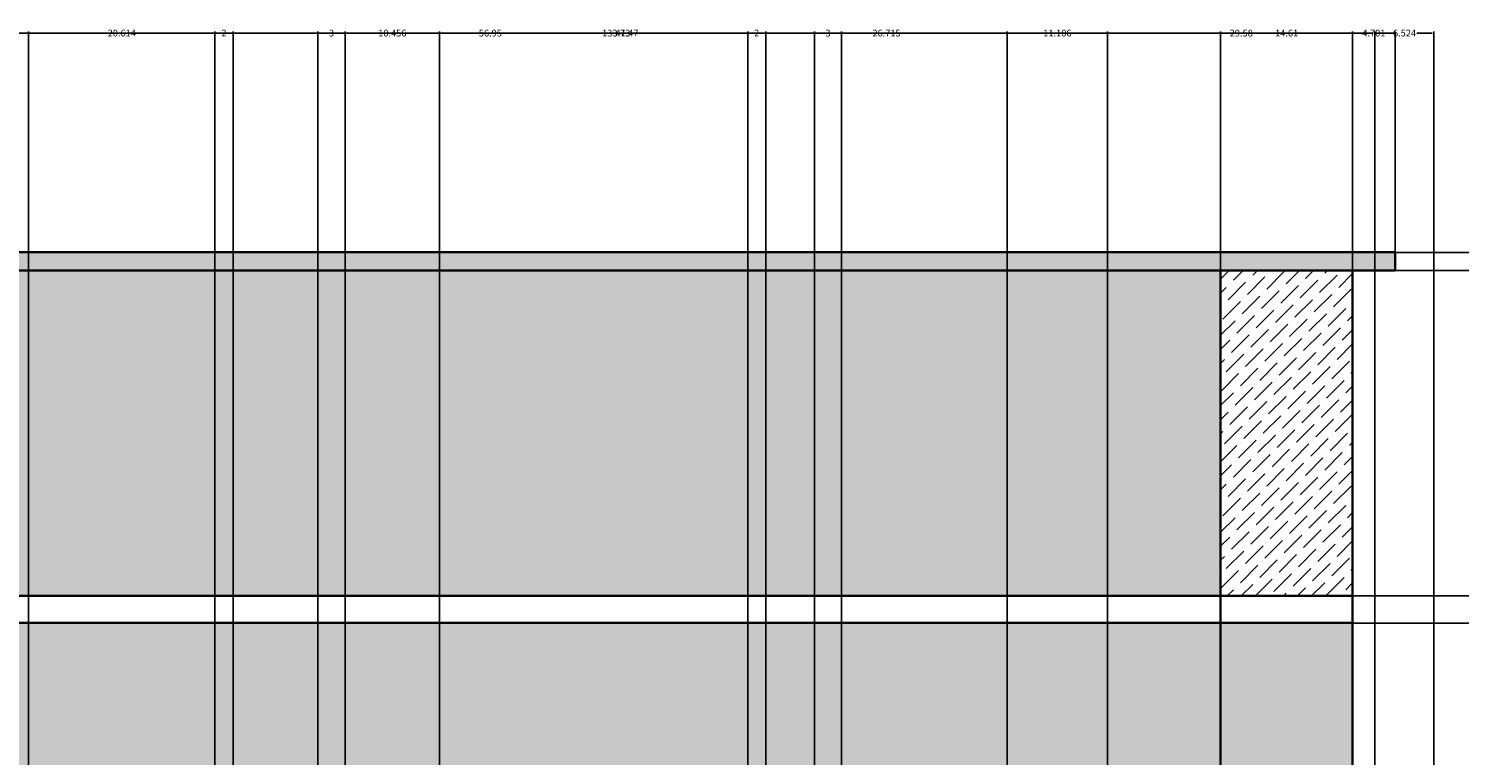
# Model space of a CAD drawing. Units: inches. Extents: x 62 to 566, y 66 to 528.
# Tile 18 of 20: x 284 to 443, y 447 to 528. Entities that reach past the tile are written whole.
import ezdxf

# ---------------------------------------------------------------- set-up
doc = ezdxf.new("R2010")
doc.units = ezdxf.units.IN
doc.header["$MEASUREMENT"] = 0
for name, color, linetype, lineweight in [('A-ANNO-DIMS', 2, 'Continuous', 18), ('A-ELEV', 7, 'Continuous', 35), ('A-WALL-PATT', 8, 'Continuous', 13)]:
    doc.layers.add(name, color=color, linetype=linetype, lineweight=lineweight)
doc.styles.get("Standard").update_dxf_attribs({"font": 'arial.ttf'})
doc.dimstyles.get("Standard").update_dxf_attribs({"dimtxt": 0.75, "dimasz": 0.18, "dimexe": 0.18, "dimexo": 0.0625, "dimgap": 0.09, "dimtad": 0, "dimtih": 1, "dimtoh": 1, "dimdec": 4, "dimzin": 0, "dimdsep": 46, "dimlunit": 4, "dimtxsty": 'Standard', "dimcen": 0.09, "dimadec": 0, "dimazin": 0, "dimtfac": 1, "dimtdec": 4, "dimtofl": 0, "dimtmove": 0, "dimatfit": 3, "dimfxl": 1, "dimtolj": 1, "dimtzin": 0, "dimarcsym": 0})

# ---------------------------------------------------------------- blocks, each defined once
blk = doc.blocks.new('*D32')
at = {"layer": 'A-ANNO-DIMS', "color": 0, "lineweight": -2, "transparency": 16777216}
for p, q in [((282.35, 501.1), (282.35, 527.47)), ((282.53, 527.29), (347.61, 527.29)), ((415.9, 527.29), (350.83, 527.29)), ((416.08, 501.1), (416.08, 527.47))]:
    blk.add_line(p, q, dxfattribs=at)
at = {"layer": 'A-ANNO-DIMS', "color": 0, "transparency": 16777216}
for points in [[(282.53, 527.32), (282.53, 527.26), (282.35, 527.29)], [(415.9, 527.32), (415.9, 527.26), (416.08, 527.29)]]:
    blk.add_solid(points, dxfattribs=at)
at = {"layer": 'Defpoints', "color": 0, "transparency": 16777216}
for p in [(416.08, 527.29), (282.35, 501.04), (416.08, 501.04)]:
    blk.add_point(p, dxfattribs=at)
at = {"layer": 'A-ANNO-DIMS', "color": 0, "transparency": 16777216, "insert": (349.22, 527.29), "char_height": 0.75, "attachment_point": 5}
blk.add_mtext('\\A1;133.73', dxfattribs=at)
blk = doc.blocks.new('*D33')
at = {"layer": 'A-ANNO-DIMS', "color": 0, "lineweight": -2, "transparency": 16777216}
for p, q in [((416.08, 501.1), (416.08, 527.47)), ((416.26, 527.29), (422.14, 527.29)), ((430.51, 527.29), (424.64, 527.29)), ((430.69, 501.1), (430.69, 527.47))]:
    blk.add_line(p, q, dxfattribs=at)
at = {"layer": 'A-ANNO-DIMS', "color": 0, "transparency": 16777216}
for points in [[(416.26, 527.32), (416.26, 527.26), (416.08, 527.29)], [(430.51, 527.32), (430.51, 527.26), (430.69, 527.29)]]:
    blk.add_solid(points, dxfattribs=at)
at = {"layer": 'Defpoints', "color": 0, "transparency": 16777216}
for p in [(430.69, 527.29), (416.08, 501.04), (430.69, 501.04)]:
    blk.add_point(p, dxfattribs=at)
at = {"layer": 'A-ANNO-DIMS', "color": 0, "transparency": 16777216, "insert": (423.39, 527.29), "char_height": 0.75, "attachment_point": 5}
blk.add_mtext('\\A1;14.61', dxfattribs=at)
blk = doc.blocks.new('*D34')
at = {"layer": 'A-ANNO-DIMS', "color": 0, "lineweight": -2, "transparency": 16777216}
for p, q in [((430.69, 501.1), (430.69, 527.47)), ((430.87, 527.29), (431.75, 527.29)), ((435.21, 527.29), (434.34, 527.29)), ((435.39, 503.1), (435.39, 527.47))]:
    blk.add_line(p, q, dxfattribs=at)
at = {"layer": 'A-ANNO-DIMS', "color": 0, "transparency": 16777216}
for points in [[(430.87, 527.32), (430.87, 527.26), (430.69, 527.29)], [(435.21, 527.32), (435.21, 527.26), (435.39, 527.29)]]:
    blk.add_solid(points, dxfattribs=at)
at = {"layer": 'Defpoints', "color": 0, "transparency": 16777216}
for p in [(435.39, 527.29), (435.39, 503.04), (430.69, 501.04)]:
    blk.add_point(p, dxfattribs=at)
at = {"layer": 'A-ANNO-DIMS', "color": 0, "transparency": 16777216, "insert": (433.04, 527.29), "char_height": 0.75, "attachment_point": 5}
blk.add_mtext('\\A1;4.701', dxfattribs=at)
blk = doc.blocks.new('*D53')
at = {"layer": 'A-ANNO-DIMS', "color": 0, "lineweight": -2, "transparency": 16777216}
for p, q in [((430.76, 462.04), (564.47, 462.04)), ((564.29, 461.86), (564.29, 454.05)), ((564.29, 445.29), (564.29, 453.1)), ((430.76, 445.11), (564.47, 445.11))]:
    blk.add_line(p, q, dxfattribs=at)
at = {"layer": 'A-ANNO-DIMS', "color": 0, "transparency": 16777216}
for points in [[(564.26, 461.86), (564.32, 461.86), (564.29, 462.04)], [(564.26, 445.29), (564.32, 445.29), (564.29, 445.11)]]:
    blk.add_solid(points, dxfattribs=at)
at = {"layer": 'Defpoints', "color": 0, "transparency": 16777216}
for p in [(430.69, 462.04), (564.29, 462.04), (430.69, 445.11)]:
    blk.add_point(p, dxfattribs=at)
at = {"layer": 'A-ANNO-DIMS', "color": 0, "transparency": 16777216, "insert": (564.29, 453.57), "char_height": 0.75, "attachment_point": 5}
blk.add_mtext('\\A1;16.936', dxfattribs=at)
blk = doc.blocks.new('*D54')
at = {"layer": 'A-ANNO-DIMS', "color": 0, "lineweight": -2, "transparency": 16777216}
for p, q in [((430.76, 465.04), (564.47, 465.04)), ((564.29, 464.86), (564.29, 464.02)), ((564.29, 462.22), (564.29, 463.07)), ((430.76, 462.04), (564.47, 462.04))]:
    blk.add_line(p, q, dxfattribs=at)
at = {"layer": 'A-ANNO-DIMS', "color": 0, "transparency": 16777216}
for points in [[(564.26, 464.86), (564.32, 464.86), (564.29, 465.04)], [(564.26, 462.22), (564.32, 462.22), (564.29, 462.04)]]:
    blk.add_solid(points, dxfattribs=at)
at = {"layer": 'Defpoints', "color": 0, "transparency": 16777216}
for p in [(430.69, 465.04), (564.29, 465.04), (430.69, 462.04)]:
    blk.add_point(p, dxfattribs=at)
at = {"layer": 'A-ANNO-DIMS', "color": 0, "transparency": 16777216, "insert": (564.29, 463.54), "char_height": 0.75, "attachment_point": 5}
blk.add_mtext('\\A1;3', dxfattribs=at)
blk = doc.blocks.new('*D55')
at = {"layer": 'A-ANNO-DIMS', "color": 0, "lineweight": -2, "transparency": 16777216}
for p, q in [((430.76, 501.04), (564.47, 501.04)), ((564.29, 500.86), (564.29, 483.52)), ((564.29, 465.22), (564.29, 482.57)), ((430.76, 465.04), (564.47, 465.04))]:
    blk.add_line(p, q, dxfattribs=at)
at = {"layer": 'A-ANNO-DIMS', "color": 0, "transparency": 16777216}
for points in [[(564.26, 500.86), (564.32, 500.86), (564.29, 501.04)], [(564.26, 465.22), (564.32, 465.22), (564.29, 465.04)]]:
    blk.add_solid(points, dxfattribs=at)
at = {"layer": 'Defpoints', "color": 0, "transparency": 16777216}
for p in [(430.69, 501.04), (564.29, 501.04), (430.69, 465.04)]:
    blk.add_point(p, dxfattribs=at)
at = {"layer": 'A-ANNO-DIMS', "color": 0, "transparency": 16777216, "insert": (564.29, 483.04), "char_height": 0.75, "attachment_point": 5}
blk.add_mtext('\\A1;36', dxfattribs=at)
blk = doc.blocks.new('*D56')
at = {"layer": 'A-ANNO-DIMS', "color": 0, "lineweight": -2, "transparency": 16777216}
for p, q in [((435.46, 503.04), (564.47, 503.04)), ((564.29, 502.86), (564.29, 502.51)), ((430.76, 501.04), (564.47, 501.04)), ((564.29, 501.22), (564.29, 501.58))]:
    blk.add_line(p, q, dxfattribs=at)
at = {"layer": 'A-ANNO-DIMS', "color": 0, "transparency": 16777216}
for points in [[(564.26, 502.86), (564.32, 502.86), (564.29, 503.04)], [(564.26, 501.22), (564.32, 501.22), (564.29, 501.04)]]:
    blk.add_solid(points, dxfattribs=at)
at = {"layer": 'Defpoints', "color": 0, "transparency": 16777216}
for p in [(435.39, 503.04), (564.29, 503.04), (430.69, 501.04)]:
    blk.add_point(p, dxfattribs=at)
at = {"layer": 'A-ANNO-DIMS', "color": 0, "transparency": 16777216, "insert": (564.29, 502.04), "char_height": 0.75, "attachment_point": 5}
blk.add_mtext('\\A1;2', dxfattribs=at)
blk = doc.blocks.new('*D61')
at = {"layer": 'A-ANNO-DIMS', "color": 0, "lineweight": -2, "transparency": 16777216}
for p, q in [((316.21, 236.72), (316.21, 527.47)), ((316.39, 527.29), (317.37, 527.29)), ((319.03, 527.29), (318.05, 527.29)), ((319.21, 233.72), (319.21, 527.47))]:
    blk.add_line(p, q, dxfattribs=at)
at = {"layer": 'A-ANNO-DIMS', "color": 0, "transparency": 16777216}
for points in [[(316.39, 527.32), (316.39, 527.26), (316.21, 527.29)], [(319.03, 527.32), (319.03, 527.26), (319.21, 527.29)]]:
    blk.add_solid(points, dxfattribs=at)
at = {"layer": 'Defpoints', "color": 0, "transparency": 16777216}
for p in [(319.21, 527.29), (316.21, 236.66), (319.21, 233.66)]:
    blk.add_point(p, dxfattribs=at)
at = {"layer": 'A-ANNO-DIMS', "color": 0, "transparency": 16777216, "insert": (317.71, 527.29), "char_height": 0.75, "attachment_point": 5}
blk.add_mtext('\\A1;3', dxfattribs=at)
blk = doc.blocks.new('*D62')
at = {"layer": 'A-ANNO-DIMS', "color": 0, "lineweight": -2, "transparency": 16777216}
for p, q in [((319.21, 233.72), (319.21, 527.47)), ((319.39, 527.29), (322.83, 527.29)), ((329.49, 527.29), (326.05, 527.29)), ((329.67, 219.79), (329.67, 527.47))]:
    blk.add_line(p, q, dxfattribs=at)
at = {"layer": 'A-ANNO-DIMS', "color": 0, "transparency": 16777216}
for points in [[(319.39, 527.32), (319.39, 527.26), (319.21, 527.29)], [(329.49, 527.32), (329.49, 527.26), (329.67, 527.29)]]:
    blk.add_solid(points, dxfattribs=at)
at = {"layer": 'Defpoints', "color": 0, "transparency": 16777216}
for p in [(329.67, 527.29), (319.21, 233.66), (329.67, 219.73)]:
    blk.add_point(p, dxfattribs=at)
at = {"layer": 'A-ANNO-DIMS', "color": 0, "transparency": 16777216, "insert": (324.44, 527.29), "char_height": 0.75, "attachment_point": 5}
blk.add_mtext('\\A1;10.456', dxfattribs=at)
blk = doc.blocks.new('*D63')
at = {"layer": 'A-ANNO-DIMS', "color": 0, "lineweight": -2, "transparency": 16777216}
for p, q in [((329.67, 219.79), (329.67, 527.47)), ((329.85, 527.29), (349.03, 527.29)), ((370.96, 527.29), (351.77, 527.29)), ((371.14, 233.72), (371.14, 527.47))]:
    blk.add_line(p, q, dxfattribs=at)
at = {"layer": 'A-ANNO-DIMS', "color": 0, "transparency": 16777216}
for points in [[(329.85, 527.32), (329.85, 527.26), (329.67, 527.29)], [(370.96, 527.32), (370.96, 527.26), (371.14, 527.29)]]:
    blk.add_solid(points, dxfattribs=at)
at = {"layer": 'Defpoints', "color": 0, "transparency": 16777216}
for p in [(371.14, 527.29), (371.14, 233.66), (329.67, 219.73)]:
    blk.add_point(p, dxfattribs=at)
at = {"layer": 'A-ANNO-DIMS', "color": 0, "transparency": 16777216, "insert": (350.4, 527.29), "char_height": 0.75, "attachment_point": 5}
blk.add_mtext('\\A1;41.47', dxfattribs=at)
blk = doc.blocks.new('*D64')
at = {"layer": 'A-ANNO-DIMS', "color": 0, "lineweight": -2, "transparency": 16777216}
for p, q in [((371.14, 233.72), (371.14, 527.47)), ((371.32, 527.29), (372.3, 527.29)), ((373.96, 527.29), (372.97, 527.29)), ((374.14, 236.72), (374.14, 527.47))]:
    blk.add_line(p, q, dxfattribs=at)
at = {"layer": 'A-ANNO-DIMS', "color": 0, "transparency": 16777216}
for points in [[(371.32, 527.32), (371.32, 527.26), (371.14, 527.29)], [(373.96, 527.32), (373.96, 527.26), (374.14, 527.29)]]:
    blk.add_solid(points, dxfattribs=at)
at = {"layer": 'Defpoints', "color": 0, "transparency": 16777216}
for p in [(374.14, 527.29), (374.14, 236.66), (371.14, 233.66)]:
    blk.add_point(p, dxfattribs=at)
at = {"layer": 'A-ANNO-DIMS', "color": 0, "transparency": 16777216, "insert": (372.64, 527.29), "char_height": 0.75, "attachment_point": 5}
blk.add_mtext('\\A1;3', dxfattribs=at)
blk = doc.blocks.new('*D74')
at = {"layer": 'A-ANNO-DIMS', "color": 0, "lineweight": -2, "transparency": 16777216}
for p, q in [((284.2, 342.84), (284.2, 527.47)), ((284.38, 527.29), (292.86, 527.29)), ((304.64, 527.29), (296.16, 527.29)), ((304.82, 342.84), (304.82, 527.47))]:
    blk.add_line(p, q, dxfattribs=at)
at = {"layer": 'A-ANNO-DIMS', "color": 0, "transparency": 16777216}
for points in [[(284.38, 527.32), (284.38, 527.26), (284.2, 527.29)], [(304.64, 527.32), (304.64, 527.26), (304.82, 527.29)]]:
    blk.add_solid(points, dxfattribs=at)
at = {"layer": 'Defpoints', "color": 0, "transparency": 16777216}
for p in [(304.82, 527.29), (284.2, 342.78), (304.82, 342.78)]:
    blk.add_point(p, dxfattribs=at)
at = {"layer": 'A-ANNO-DIMS', "color": 0, "transparency": 16777216, "insert": (294.51, 527.29), "char_height": 0.75, "attachment_point": 5}
blk.add_mtext('\\A1;20.614', dxfattribs=at)
blk = doc.blocks.new('*D75')
at = {"layer": 'A-ANNO-DIMS', "color": 0, "lineweight": -2, "transparency": 16777216}
for p, q in [((304.82, 342.84), (304.82, 527.47)), ((305, 527.29), (305.48, 527.29)), ((306.64, 527.29), (306.15, 527.29)), ((306.82, 342.84), (306.82, 527.47))]:
    blk.add_line(p, q, dxfattribs=at)
at = {"layer": 'A-ANNO-DIMS', "color": 0, "transparency": 16777216}
for points in [[(305, 527.32), (305, 527.26), (304.82, 527.29)], [(306.64, 527.32), (306.64, 527.26), (306.82, 527.29)]]:
    blk.add_solid(points, dxfattribs=at)
at = {"layer": 'Defpoints', "color": 0, "transparency": 16777216}
for p in [(306.82, 527.29), (304.82, 342.78), (306.82, 342.78)]:
    blk.add_point(p, dxfattribs=at)
at = {"layer": 'A-ANNO-DIMS', "color": 0, "transparency": 16777216, "insert": (305.82, 527.29), "char_height": 0.75, "attachment_point": 5}
blk.add_mtext('\\A1;2', dxfattribs=at)
blk = doc.blocks.new('*D76')
at = {"layer": 'A-ANNO-DIMS', "color": 0, "lineweight": -2, "transparency": 16777216}
for p, q in [((306.82, 342.84), (306.82, 527.47)), ((307, 527.29), (333.93, 527.29)), ((363.58, 527.29), (336.65, 527.29)), ((363.76, 342.84), (363.76, 527.47))]:
    blk.add_line(p, q, dxfattribs=at)
at = {"layer": 'A-ANNO-DIMS', "color": 0, "transparency": 16777216}
for points in [[(307, 527.32), (307, 527.26), (306.82, 527.29)], [(363.58, 527.32), (363.58, 527.26), (363.76, 527.29)]]:
    blk.add_solid(points, dxfattribs=at)
at = {"layer": 'Defpoints', "color": 0, "transparency": 16777216}
for p in [(363.76, 527.29), (306.82, 342.78), (363.76, 342.78)]:
    blk.add_point(p, dxfattribs=at)
at = {"layer": 'A-ANNO-DIMS', "color": 0, "transparency": 16777216, "insert": (335.29, 527.29), "char_height": 0.75, "attachment_point": 5}
blk.add_mtext('\\A1;56.95', dxfattribs=at)
blk = doc.blocks.new('*D77')
at = {"layer": 'A-ANNO-DIMS', "color": 0, "lineweight": -2, "transparency": 16777216}
for p, q in [((363.76, 342.84), (363.76, 527.47)), ((363.94, 527.29), (364.43, 527.29)), ((365.58, 527.29), (365.1, 527.29)), ((365.76, 342.84), (365.76, 527.47))]:
    blk.add_line(p, q, dxfattribs=at)
at = {"layer": 'A-ANNO-DIMS', "color": 0, "transparency": 16777216}
for points in [[(363.94, 527.32), (363.94, 527.26), (363.76, 527.29)], [(365.58, 527.32), (365.58, 527.26), (365.76, 527.29)]]:
    blk.add_solid(points, dxfattribs=at)
at = {"layer": 'Defpoints', "color": 0, "transparency": 16777216}
for p in [(365.76, 527.29), (363.76, 342.78), (365.76, 342.78)]:
    blk.add_point(p, dxfattribs=at)
at = {"layer": 'A-ANNO-DIMS', "color": 0, "transparency": 16777216, "insert": (364.76, 527.29), "char_height": 0.75, "attachment_point": 5}
blk.add_mtext('\\A1;2', dxfattribs=at)
blk = doc.blocks.new('*D78')
at = {"layer": 'A-ANNO-DIMS', "color": 0, "lineweight": -2, "transparency": 16777216}
for p, q in [((365.76, 342.84), (365.76, 527.47)), ((365.94, 527.29), (377.47, 527.29)), ((392.3, 527.29), (380.78, 527.29)), ((392.48, 342.84), (392.48, 527.47))]:
    blk.add_line(p, q, dxfattribs=at)
at = {"layer": 'A-ANNO-DIMS', "color": 0, "transparency": 16777216}
for points in [[(365.94, 527.32), (365.94, 527.26), (365.76, 527.29)], [(392.3, 527.32), (392.3, 527.26), (392.48, 527.29)]]:
    blk.add_solid(points, dxfattribs=at)
at = {"layer": 'Defpoints', "color": 0, "transparency": 16777216}
for p in [(392.48, 527.29), (365.76, 342.78), (392.48, 342.78)]:
    blk.add_point(p, dxfattribs=at)
at = {"layer": 'A-ANNO-DIMS', "color": 0, "transparency": 16777216, "insert": (379.12, 527.29), "char_height": 0.75, "attachment_point": 5}
blk.add_mtext('\\A1;26.715', dxfattribs=at)
blk = doc.blocks.new('*D79')
at = {"layer": 'A-ANNO-DIMS', "color": 0, "lineweight": -2, "transparency": 16777216}
for p, q in [((392.48, 352.55), (392.48, 527.47)), ((392.66, 527.29), (396.42, 527.29)), ((403.4, 527.29), (399.64, 527.29)), ((403.58, 340.55), (403.58, 527.47))]:
    blk.add_line(p, q, dxfattribs=at)
at = {"layer": 'A-ANNO-DIMS', "color": 0, "transparency": 16777216}
for points in [[(392.66, 527.32), (392.66, 527.26), (392.48, 527.29)], [(403.4, 527.32), (403.4, 527.26), (403.58, 527.29)]]:
    blk.add_solid(points, dxfattribs=at)
at = {"layer": 'Defpoints', "color": 0, "transparency": 16777216}
for p in [(403.58, 527.29), (392.48, 352.48), (403.58, 340.49)]:
    blk.add_point(p, dxfattribs=at)
at = {"layer": 'A-ANNO-DIMS', "color": 0, "transparency": 16777216, "insert": (398.03, 527.29), "char_height": 0.75, "attachment_point": 5}
blk.add_mtext('\\A1;11.106', dxfattribs=at)
blk = doc.blocks.new('*D80')
at = {"layer": 'A-ANNO-DIMS', "color": 0, "lineweight": -2, "transparency": 16777216}
for p, q in [((403.58, 340.55), (403.58, 527.47)), ((403.76, 527.29), (417.01, 527.29)), ((432.98, 527.29), (419.74, 527.29)), ((433.16, 340.55), (433.16, 527.47))]:
    blk.add_line(p, q, dxfattribs=at)
at = {"layer": 'A-ANNO-DIMS', "color": 0, "transparency": 16777216}
for points in [[(403.76, 527.32), (403.76, 527.26), (403.58, 527.29)], [(432.98, 527.32), (432.98, 527.26), (433.16, 527.29)]]:
    blk.add_solid(points, dxfattribs=at)
at = {"layer": 'Defpoints', "color": 0, "transparency": 16777216}
for p in [(433.16, 527.29), (403.58, 340.49), (433.16, 340.49)]:
    blk.add_point(p, dxfattribs=at)
at = {"layer": 'A-ANNO-DIMS', "color": 0, "transparency": 16777216, "insert": (418.37, 527.29), "char_height": 0.75, "attachment_point": 5}
blk.add_mtext('\\A1;29.58', dxfattribs=at)
blk = doc.blocks.new('*D81')
at = {"layer": 'A-ANNO-DIMS', "color": 0, "lineweight": -2, "transparency": 16777216}
for p, q in [((433.16, 340.55), (433.16, 527.47)), ((433.34, 527.29), (435.07, 527.29)), ((439.51, 527.29), (437.78, 527.29)), ((439.69, 352.55), (439.69, 527.47))]:
    blk.add_line(p, q, dxfattribs=at)
at = {"layer": 'A-ANNO-DIMS', "color": 0, "transparency": 16777216}
for points in [[(433.34, 527.32), (433.34, 527.26), (433.16, 527.29)], [(439.51, 527.32), (439.51, 527.26), (439.69, 527.29)]]:
    blk.add_solid(points, dxfattribs=at)
at = {"layer": 'Defpoints', "color": 0, "transparency": 16777216}
for p in [(439.69, 527.29), (439.69, 352.48), (433.16, 340.49)]:
    blk.add_point(p, dxfattribs=at)
at = {"layer": 'A-ANNO-DIMS', "color": 0, "transparency": 16777216, "insert": (436.43, 527.29), "char_height": 0.75, "attachment_point": 5}
blk.add_mtext('\\A1;6.524', dxfattribs=at)

msp = doc.modelspace()

# ---------------------------------------------------------------- hatches: boundary and pattern name
at = {"layer": 'A-WALL-PATT'}
h = msp.add_hatch(color=256, dxfattribs=at)
h.dxf.hatch_style = 1
h.paths.add_polyline_path([(416.0836, 462.0423), (125.9418, 462.0423), (125.9418, 414.3686), (125.9418, 270.3686), (125.9418, 126.3686), (142.3851, 126.3686), (142.3851, 270.3686), (142.3851, 414.3686), (142.3851, 445.1064), (284.2021, 445.1064), (416.0836, 445.1064)])
h.paths.add_polyline_path([(435.3945, 503.0423), (426.3652, 503.0423), (120.4058, 503.0423), (120.4058, 501.0423), (125.9418, 501.0423), (416.0836, 501.0423), (426.3652, 501.0423), (430.6938, 501.0423), (435.3945, 501.0423)])
h.paths.add_polyline_path([(439.6878, 352.4848), (392.4793, 352.4848), (392.4793, 307.4128), (217.2752, 307.4128), (217.2752, 295.4098), (217.2752, 271.4128), (272.0586, 271.4128), (439.6878, 271.4128)])
h.paths.add_polyline_path([(248.0143, 297.1682), (255.6783, 297.1682), (255.6783, 280.0423), (248.0143, 280.0423)], flags=16)
h.paths.add_polyline_path([(235.4641, 280.0423), (227.8001, 280.0423), (227.8001, 297.1682), (235.4641, 297.1682)], flags=16)
h.paths.add_polyline_path([(270.4427, 297.1682), (278.1067, 297.1682), (278.1067, 280.0423), (270.4427, 280.0423)], flags=16)
h.paths.add_polyline_path([(296.3755, 297.1682), (304.0395, 297.1682), (304.0395, 280.0423), (296.3755, 280.0423)], flags=16)
h.paths.add_polyline_path([(319.2543, 297.1682), (326.9183, 297.1682), (326.9183, 280.0423), (319.2543, 280.0423)], flags=16)
h.paths.add_polyline_path([(341.2622, 297.1682), (348.9262, 297.1682), (348.9262, 280.0423), (341.2622, 280.0423)], flags=16)
h.paths.add_polyline_path([(389.2857, 298.3985), (433.8102, 298.3985), (433.8102, 294.9497), (389.2857, 294.9497)], flags=16)
h.paths.add_polyline_path([(389.2857, 291.6038), (433.8102, 291.6038), (433.8102, 288.155), (389.2857, 288.155)], flags=16)
h.paths.add_polyline_path([(389.2857, 284.9607), (433.8102, 284.9607), (433.8102, 281.5119), (389.2857, 281.5119)], flags=16)
h.paths.add_polyline_path([(403.5849, 311.4736), (403.5849, 317.4388), (433.1636, 317.4388), (433.1636, 311.4736)], flags=16)
h.paths.add_polyline_path([(403.5849, 323.1329), (403.5849, 329.0982), (433.1636, 329.0982), (433.1636, 323.1329)], flags=16)
h.paths.add_polyline_path([(403.5849, 334.5211), (403.5849, 340.4863), (433.1636, 340.4863), (433.1636, 334.5211)], flags=16)
h.paths.add_polyline_path([(272.0586, 160.3545), (217.2752, 160.3545), (217.2752, 129.0504), (217.2752, 126.3686), (272.0586, 126.3686)], flags=17)
h.paths.add_polyline_path([(220.5897, 149.5749), (220.5897, 152.296), (267.7931, 152.296), (267.7931, 149.5749)], flags=16)
h.paths.add_polyline_path([(267.7931, 146.6724), (267.7931, 143.9513), (220.5897, 143.9513), (220.5897, 146.6724)], flags=16)
h.paths.add_polyline_path([(220.5897, 155.3799), (220.5897, 158.101), (267.7931, 158.101), (267.7931, 155.3799)], flags=16)
h.paths.add_polyline_path([(267.7931, 140.686), (267.7931, 137.9649), (220.5897, 137.9649), (220.5897, 140.686)], flags=16)
h.paths.add_polyline_path([(267.7931, 135.516), (267.7931, 132.7949), (220.5897, 132.7949), (220.5897, 135.516)], flags=16)
h = msp.add_hatch(color=256, dxfattribs=at)
h.dxf.hatch_style = 1
h.paths.add_polyline_path([(416.0836, 501.0423), (282.3509, 501.0423), (282.3509, 465.0423), (416.0836, 465.0423)])
h.paths.add_polyline_path([(284.2021, 420.597), (272.0586, 420.597), (272.0586, 309.5388), (272.0586, 307.4128), (284.2021, 307.4128)], flags=17)
h.paths.add_polyline_path([(284.2021, 445.1064), (142.3851, 445.1064), (142.3851, 414.3686), (142.3851, 270.3686), (142.3851, 126.3686), (163.6548, 126.3686), (163.6548, 270.5016), (163.6548, 414.5016), (163.6548, 427.4752), (284.2021, 427.4752)])
h.paths.add_polyline_path([(235.4641, 297.1682), (227.8001, 297.1682), (227.8001, 280.0423), (235.4641, 280.0423)], flags=17)
h.paths.add_polyline_path([(255.6783, 297.1682), (248.0143, 297.1682), (248.0143, 280.0423), (255.6783, 280.0423)], flags=17)
h.paths.add_polyline_path([(278.1067, 297.1682), (270.4427, 297.1682), (270.4427, 280.0423), (278.1067, 280.0423)], flags=17)
h.paths.add_polyline_path([(304.0395, 297.1682), (296.3755, 297.1682), (296.3755, 280.0423), (304.0395, 280.0423)])
h.paths.add_polyline_path([(326.9183, 297.1682), (319.2543, 297.1682), (319.2543, 280.0423), (326.9183, 280.0423)])
h.paths.add_polyline_path([(348.9262, 297.1682), (341.2622, 297.1682), (341.2622, 280.0423), (348.9262, 280.0423)])
h.paths.add_polyline_path([(433.8102, 284.9607), (389.2857, 284.9607), (389.2857, 281.5119), (433.8102, 281.5119)])
h.paths.add_polyline_path([(433.8102, 291.6038), (389.2857, 291.6038), (389.2857, 288.155), (433.8102, 288.155)])
h.paths.add_polyline_path([(433.8102, 298.3985), (389.2857, 298.3985), (389.2857, 294.9497), (433.8102, 294.9497)])
h.paths.add_polyline_path([(433.1636, 317.4388), (403.5849, 317.4388), (403.5849, 311.4736), (433.1636, 311.4736)])
h.paths.add_polyline_path([(433.1636, 329.0982), (403.5849, 329.0982), (403.5849, 323.1329), (433.1636, 323.1329)])
h.paths.add_polyline_path([(433.1636, 340.4863), (403.5849, 340.4863), (403.5849, 334.5211), (433.1636, 334.5211)])
h.paths.add_polyline_path([(284.2021, 271.4128), (272.0586, 271.4128), (272.0586, 160.3545), (272.0586, 126.3686), (284.2021, 126.3686)])
h.paths.add_polyline_path([(267.7931, 158.101), (220.5897, 158.101), (220.5897, 155.3799), (267.7931, 155.3799)], flags=17)
h.paths.add_polyline_path([(267.7931, 152.296), (220.5897, 152.296), (220.5897, 149.5749), (267.7931, 149.5749)], flags=17)
h.paths.add_polyline_path([(267.7931, 146.6724), (220.5897, 146.6724), (220.5897, 143.9513), (267.7931, 143.9513)], flags=17)
h.paths.add_polyline_path([(267.7931, 140.686), (220.5897, 140.686), (220.5897, 137.9649), (267.7931, 137.9649)], flags=17)
h.paths.add_polyline_path([(267.7931, 135.516), (220.5897, 135.516), (220.5897, 132.7949), (267.7931, 132.7949)], flags=17)
h.paths.add_polyline_path([(148.2354, 493.4274), (140.5713, 493.4274), (140.5713, 476.3015), (148.2354, 476.3015)])
h.paths.add_polyline_path([(163.2545, 493.4274), (155.5905, 493.4274), (155.5905, 476.3015), (163.2545, 476.3015)])
h.paths.add_polyline_path([(177.9243, 493.7764), (170.2603, 493.7764), (170.2603, 476.6506), (177.9243, 476.6506)])
h.paths.add_polyline_path([(193.9913, 493.7764), (186.3273, 493.7764), (186.3273, 476.6506), (193.9913, 476.6506)])
h.paths.add_polyline_path([(209.709, 493.7764), (202.045, 493.7764), (202.045, 476.6506), (209.709, 476.6506)])
h = msp.add_hatch(dxfattribs=at)
h.set_pattern_fill('ANSI36', color=256, scale=8.8)
h.paths.add_polyline_path([(430.6938, 501.0423), (426.3652, 501.0423), (416.0836, 501.0423), (416.0836, 465.0423), (430.6938, 465.0423)])
h = msp.add_hatch(color=256, dxfattribs=at)
h.dxf.hatch_style = 1
h.paths.add_polyline_path([(430.6938, 462.0423), (416.0836, 462.0423), (416.0836, 445.1064), (430.6938, 445.1064)])
h.paths.add_polyline_path([(169.0431, 420.597), (284.2021, 420.597), (284.2021, 426.4752), (164.6548, 426.4752), (164.6548, 414.5016), (164.6548, 126.3686), (169.0431, 126.3686)])

# ---------------------------------------------------------------- linework, layer by layer
at = {"layer": 'A-ELEV'}
for p, q in [((120.4058, 503.0423), (426.3652, 503.0423)), ((426.3652, 503.0423), (435.3945, 503.0423)), ((435.3945, 503.0423), (435.3945, 501.0423)), ((125.9418, 501.0423), (416.0836, 501.0423)), ((416.0836, 501.0423), (416.0836, 465.0423)), ((426.3652, 501.0423), (416.0836, 501.0423)), ((430.6938, 501.0423), (426.3652, 501.0423)), ((430.6938, 465.0423), (430.6938, 501.0423)), ((435.3945, 501.0423), (430.6938, 501.0423)), ((125.9418, 465.0423), (416.0836, 465.0423)), ((416.0836, 465.0423), (416.0836, 462.0423)), ((416.0836, 465.0423), (430.6938, 465.0423)), ((430.6938, 462.0423), (430.6938, 465.0423)), ((125.9418, 462.0423), (416.0836, 462.0423)), ((416.0836, 352.4848), (416.0836, 462.0423)), ((416.0836, 462.0423), (430.6938, 462.0423)), ((430.6938, 445.1064), (430.6938, 462.0423))]:
    msp.add_line(p, q, dxfattribs=at)

# ---------------------------------------------------------------- dimensions: what is measured, and where the dimension line sits
at = {"layer": 'A-ANNO-DIMS'}
for base, p1, p2, override, picture, middle in [((416.0836, 527.2923), (282.3509, 501.0423), (416.0836, 501.0423), {"dimdec": 2, "dimlfac": 1, "dimrnd": 0, "dimzin": 0, "dimdsep": 46, "dimlunit": 2}, '*D32', (349.2172, 527.2923)), ((304.8163, 527.2923), (284.2021, 342.7821), (304.8163, 342.7821), {"dimdec": 3, "dimlfac": 1, "dimrnd": 0, "dimzin": 0, "dimdsep": 46, "dimlunit": 2}, '*D74', (294.5092, 527.2923)), ((306.8163, 527.2923), (304.8163, 342.7821), (306.8163, 342.7821), {"dimdec": 0, "dimlfac": 1, "dimrnd": 0, "dimzin": 0, "dimdsep": 46, "dimlunit": 2}, '*D75', (305.8163, 527.2923)), ((363.764, 527.2923), (306.8163, 342.7821), (363.764, 342.7821), {"dimdec": 2, "dimlfac": 1, "dimrnd": 0, "dimzin": 0, "dimdsep": 46, "dimlunit": 2}, '*D76', (335.2902, 527.2923)), ((319.2101, 527.2923), (316.2101, 236.6618), (319.2101, 233.6618), {"dimdec": 0, "dimlfac": 1, "dimrnd": 0, "dimzin": 0, "dimdsep": 46, "dimlunit": 2}, '*D61', (317.7101, 527.2923)), ((329.6665, 527.2923), (319.2101, 233.6618), (329.6665, 219.7304), {"dimdec": 3, "dimlfac": 1, "dimrnd": 0, "dimzin": 0, "dimdsep": 46, "dimlunit": 2}, '*D62', (324.4383, 527.2923)), ((371.1373, 527.2923), (329.6665, 219.7304), (371.1373, 233.6618), {"dimdec": 2, "dimlfac": 1, "dimrnd": 0, "dimzin": 0, "dimdsep": 46, "dimlunit": 2}, '*D63', (350.4019, 527.2923)), ((365.764, 527.2923), (363.764, 342.7821), (365.764, 342.7821), {"dimdec": 0, "dimlfac": 1, "dimrnd": 0, "dimzin": 0, "dimdsep": 46, "dimlunit": 2}, '*D77', (364.764, 527.2923)), ((392.4793, 527.2923), (365.764, 342.7821), (392.4793, 342.7821), {"dimdec": 3, "dimlfac": 1, "dimrnd": 0, "dimzin": 0, "dimdsep": 46, "dimlunit": 2}, '*D78', (379.1216, 527.2923)), ((374.1373, 527.2923), (371.1373, 233.6618), (374.1373, 236.6618), {"dimdec": 0, "dimlfac": 1, "dimrnd": 0, "dimzin": 0, "dimdsep": 46, "dimlunit": 2}, '*D64', (372.6373, 527.2923)), ((403.5849, 527.2923), (392.4793, 352.4848), (403.5849, 340.4863), {"dimdec": 3, "dimlfac": 1, "dimrnd": 0, "dimzin": 0, "dimdsep": 46, "dimlunit": 2}, '*D79', (398.0321, 527.2923)), ((433.1636, 527.2923), (403.5849, 340.4863), (433.1636, 340.4863), {"dimdec": 2, "dimlfac": 1, "dimrnd": 0, "dimzin": 0, "dimdsep": 46, "dimlunit": 2}, '*D80', (418.3743, 527.2923)), ((430.6938, 527.2923), (416.0836, 501.0423), (430.6938, 501.0423), {"dimdec": 2, "dimlfac": 1, "dimrnd": 0, "dimzin": 0, "dimdsep": 46, "dimlunit": 2}, '*D33', (423.3887, 527.2923)), ((435.3945, 527.2923), (430.6938, 501.0423), (435.3945, 503.0423), {"dimdec": 3, "dimlfac": 1, "dimrnd": 0, "dimzin": 0, "dimdsep": 46, "dimlunit": 2}, '*D34', (433.0442, 527.2923)), ((439.6878, 527.2923), (433.1636, 340.4863), (439.6878, 352.4848), {"dimdec": 3, "dimlfac": 1, "dimrnd": 0, "dimzin": 0, "dimdsep": 46, "dimlunit": 2}, '*D81', (436.4257, 527.2923))]:
    dim = msp.add_linear_dim(base=base, p1=p1, p2=p2, dimstyle='Standard', override=override, dxfattribs=at)
    dim.commit()
    dim.dimension.update_dxf_attribs({"geometry": picture, "text_midpoint": middle})
for base, p1, p2, override, picture, middle in [((564.2868, 503.0423), (430.6938, 501.0423), (435.3945, 503.0423), {"dimdec": 0, "dimlfac": 1, "dimrnd": 0, "dimzin": 0, "dimdsep": 46, "dimlunit": 2}, '*D56', (564.2868, 502.0423)), ((564.2868, 501.0423), (430.6938, 465.0423), (430.6938, 501.0423), {"dimdec": 0, "dimlfac": 1, "dimrnd": 0, "dimzin": 0, "dimdsep": 46, "dimlunit": 2}, '*D55', (564.2868, 483.0423)), ((564.2868, 465.0423), (430.6938, 462.0423), (430.6938, 465.0423), {"dimdec": 0, "dimlfac": 1, "dimrnd": 0, "dimzin": 0, "dimdsep": 46, "dimlunit": 2}, '*D54', (564.2868, 463.5423)), ((564.2868, 462.0423), (430.6938, 445.1064), (430.6938, 462.0423), {"dimdec": 3, "dimlfac": 1, "dimrnd": 0, "dimzin": 0, "dimdsep": 46, "dimlunit": 2}, '*D53', (564.2868, 453.5744))]:
    dim = msp.add_linear_dim(base=base, p1=p1, p2=p2, angle=90, dimstyle='Standard', override=override, dxfattribs=at)
    dim.commit()
    dim.dimension.update_dxf_attribs({"geometry": picture, "text_midpoint": middle})

doc.saveas('drawing.dxf')
